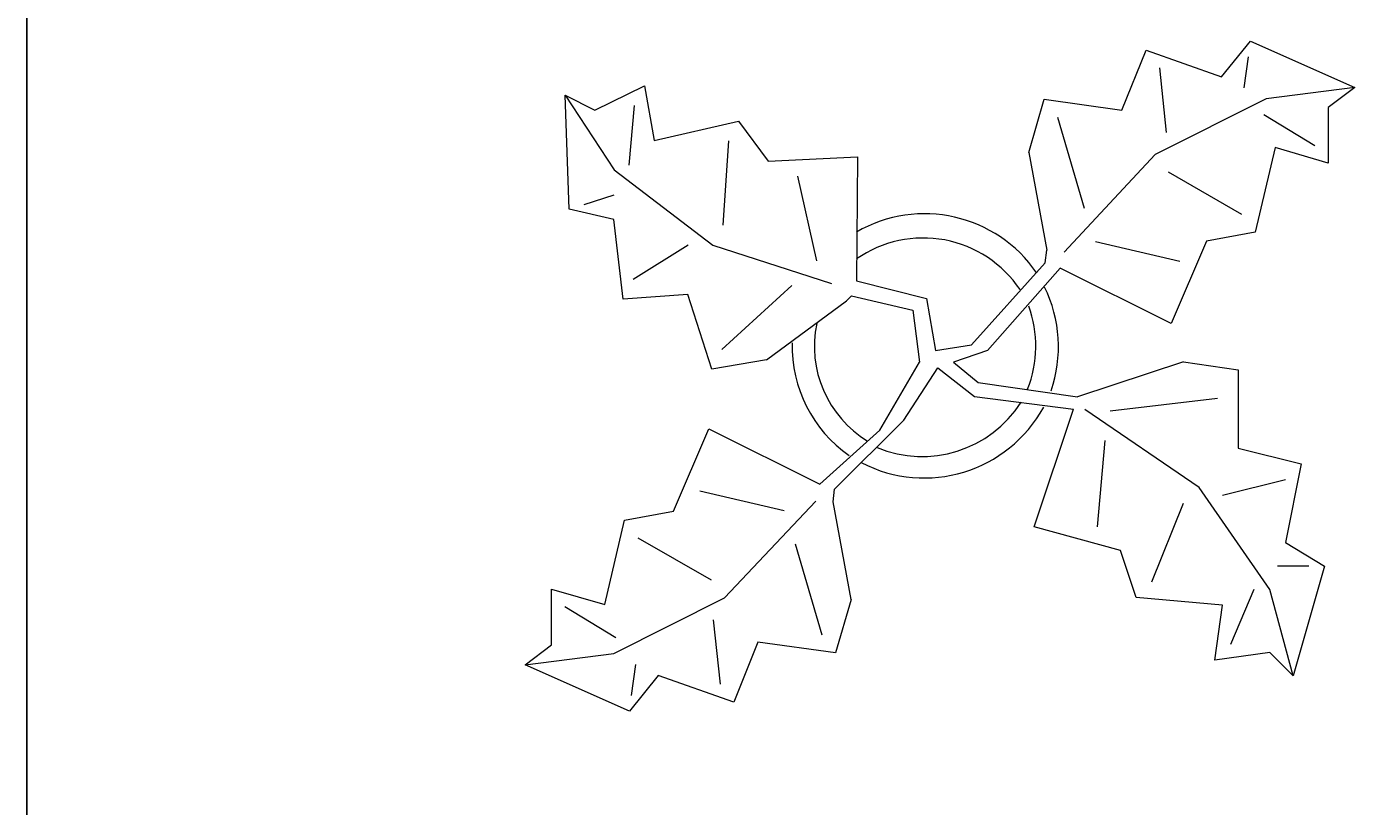
# Model space of a CAD drawing. Units: inches. Extents: x -301 to 715, y -607 to 364.
# Tile 54 of 141: x -205 to -164, y -260 to -237. Entities that reach past the tile are written whole.
import ezdxf

# ---------------------------------------------------------------- set-up
doc = ezdxf.new("R2010")
doc.units = ezdxf.units.IN
doc.header["$MEASUREMENT"] = 0
doc.layers.add('A-ANNO-DIMS', color=2, linetype='Continuous', lineweight=18)
doc.layers.add('L-PLNT', color=94, linetype='Continuous', lineweight=13)
doc.styles.get("Standard").update_dxf_attribs({"font": 'arial.ttf'})
doc.dimstyles.get("Standard").update_dxf_attribs({"dimtxt": 0.18, "dimasz": 0.18, "dimexe": 0.18, "dimexo": 0.0625, "dimgap": 0.09, "dimtad": 0, "dimtih": 1, "dimtoh": 1, "dimdec": 1, "dimzin": 0, "dimdsep": 46, "dimlunit": 4, "dimtxsty": 'Standard', "dimcen": 0.09, "dimclrd": 3, "dimclre": 4, "dimclrt": 6, "dimadec": 0, "dimazin": 0, "dimtfac": 1, "dimtdec": 1, "dimtofl": 0, "dimtmove": 0, "dimatfit": 3, "dimfxl": 1, "dimtfill": 2, "dimtfillclr": 51, "dimtolj": 1, "dimtzin": 0, "dimarcsym": 0})

# ---------------------------------------------------------------- blocks, each defined once
blk = doc.blocks.new('Plant - Rubber or Philodendron')
for p, q in [((8.8871, 10.7908), (9.9809, 13.4933)), ((9.9809, 13.4933), (13.3837, 12.301)), ((13.3837, 12.301), (14.68, 13.9039)), ((14.68, 13.9039), (19.3848, 11.8146)), ((14.5816, 13.2037), (14.3848, 11.8033)), ((10.5828, 12.6946), (10.8893, 9.7953)), ((-14.8639, 10.7964), (-12.6195, 11.8975)), ((-12.6195, 11.8975), (-12.1909, 9.4345)), ((19.3848, 11.8146), (15.3859, 11.3055)), ((19.3848, 11.8146), (18.1868, 10.9119)), ((-16.2005, 11.4774), (-13.9899, 8.1064)), ((-16.2005, 11.4774), (-14.8639, 10.7964)), ((-16.0159, 6.3329), (-16.2005, 11.4774)), ((-13.3174, 8.325), (-13.0735, 11.0065)), ((4.6914, 8.8812), (5.3859, 11.2828)), ((5.3859, 11.2828), (8.8871, 10.7908)), ((15.3859, 11.3055), (10.3916, 8.7942)), ((5.9878, 10.4842), (7.1971, 6.3869)), ((15.2875, 10.6053), (17.5907, 9.2105)), ((18.1868, 10.9119), (18.1925, 8.4119)), ((-12.1909, 9.4345), (-8.3829, 10.3)), ((-8.3829, 10.3), (-7.0549, 8.501)), ((-8.8369, 9.409), (-9.0894, 5.6095)), ((15.7909, 9.1065), (14.8995, 5.3044)), ((18.1925, 8.4119), (15.7909, 9.1065)), ((-7.0549, 8.501), (-3.0284, 8.6941)), ((-3.0284, 8.6941), (-3.0709, 3.1041)), ((4.6914, 8.8812), (5.5014, 4.4831)), ((10.3916, 8.7942), (6.2847, 4.4028)), ((-13.9899, 8.1064), (-9.5434, 4.7185)), ((14.2977, 6.1031), (10.9934, 7.9956)), ((-4.8529, 4.012), (-5.7184, 7.82)), ((-15.3434, 6.5514), (-13.9984, 6.9884)), ((-14.0069, 5.8704), (-16.0159, 6.3329)), ((-13.5868, 2.2894), (-14.0069, 5.8704)), ((7.7005, 4.8881), (11.5025, 3.9967)), ((12.7005, 4.8994), (11.1089, 1.1958)), ((14.8995, 5.3044), (12.7005, 4.8994)), ((-13.1329, 3.1804), (-10.6614, 4.727)), ((-9.5434, 4.7185), (-4.1917, 2.9888)), ((5.4346, 3.9146), (5.5014, 4.4831)), ((2.1141, 0.2298), (5.4346, 3.9146)), ((6.1032, 3.6844), (2.8262, -0.031)), ((11.1089, 1.1958), (6.1032, 3.6844)), ((-3.0709, 3.1041), (0.0797, 2.3163)), ((-10.6784, 2.491), (-13.5868, 2.2894)), ((-9.5858, -0.8715), (-10.6784, 2.491)), ((-9.1318, 0.0195), (-5.9793, 2.9025)), ((-3.5248, 2.2131), (-3.3011, 2.4355)), ((-3.3011, 2.4355), (-0.5306, 1.7947)), ((-7.1228, -0.443), (-3.5248, 2.2131)), ((0.0797, 2.3163), (0.4866, -0.031)), ((-0.5306, 1.7947), (-0.2255, -0.5527)), ((-0.5306, 1.7947), (-0.5306, 1.7947)), ((0.4866, -0.031), (2.1141, 0.2298)), ((-7.1228, -0.443), (-9.5858, -0.8715)), ((-2.019, -3.6148), (-0.2255, -0.5527)), ((2.8262, -0.031), (1.3003, -0.5527)), ((1.3003, -0.5527), (2.4193, -1.4655)), ((11.6605, -0.5413), (6.895, -2.1175)), ((11.6605, -0.5413), (14.1354, -0.8948)), ((-0.9375, -3.1608), (0.5883, -0.8135)), ((0.5883, -0.8135), (2.2447, -2.0916)), ((14.1354, -0.8948), (14.1354, -4.4304)), ((2.4193, -1.4655), (6.895, -2.1175)), ((2.2447, -2.0916), (6.7108, -2.6626)), ((8.3544, -2.7453), (13.1973, -2.1704)), ((4.943, -7.9659), (6.7108, -2.6626)), ((12.3677, -6.1981), (7.219, -2.6772)), ((-11.3237, -7.2629), (-9.7321, -3.5593)), ((-9.7321, -3.5593), (-4.7264, -6.0479)), ((-2.019, -3.6148), (-4.7264, -6.0479)), ((-4.0579, -6.2781), (-0.9375, -3.1608)), ((8.125, -4.0768), (7.7715, -7.9659)), ((14.1354, -4.4304), (16.9638, -5.1375)), ((16.9638, -5.1375), (16.2567, -8.673)), ((16.2567, -5.8446), (13.4283, -6.5517)), ((-6.3237, -7.2516), (-10.1257, -6.3602)), ((-4.1246, -6.8466), (-4.0579, -6.2781)), ((15.5496, -10.7943), (12.3677, -6.1981)), ((-13.5228, -7.6679), (-11.3237, -7.2629)), ((-9.0148, -11.1577), (-4.9047, -6.8122)), ((-3.3146, -11.2447), (-4.1246, -6.8466)), ((10.2463, -10.4408), (11.6605, -6.9053)), ((-14.4141, -11.4699), (-13.5228, -7.6679)), ((-12.921, -8.4665), (-9.6166, -10.359)), ((8.8321, -9.0266), (4.943, -7.9659)), ((-4.611, -12.8477), (-5.8203, -8.7504)), ((9.5392, -11.1479), (8.8321, -9.0266)), ((16.2567, -8.673), (18.0245, -9.7337)), ((17.3174, -9.7337), (15.9032, -9.7337)), ((18.0245, -9.7337), (16.6103, -14.6834)), ((-16.8157, -10.7754), (-14.4141, -11.4699)), ((-16.8101, -13.2754), (-16.8157, -10.7754)), ((14.8425, -10.7943), (13.7819, -13.2692)), ((16.6103, -14.6834), (15.5496, -10.7943)), ((-14.0091, -13.669), (-9.0148, -11.1577)), ((-3.3146, -11.2447), (-4.0092, -13.6463)), ((13.4283, -11.5015), (9.5392, -11.1479)), ((13.0748, -13.9763), (13.4283, -11.5015)), ((-13.9107, -12.9688), (-16.2139, -11.574)), ((-9.206, -15.0581), (-9.5126, -12.1588)), ((-18.008, -14.1781), (-16.8101, -13.2754)), ((-7.5103, -13.1543), (-8.6042, -15.8568)), ((-4.0092, -13.6463), (-7.5103, -13.1543)), ((-18.008, -14.1781), (-14.0091, -13.669)), ((15.5496, -13.6228), (13.0748, -13.9763)), ((16.6103, -14.6834), (15.5496, -13.6228)), ((-13.3032, -16.2674), (-18.008, -14.1781)), ((-13.2048, -15.5672), (-13.008, -14.1668)), ((-12.0069, -14.6645), (-13.3032, -16.2674)), ((-8.6042, -15.8568), (-12.0069, -14.6645))]:
    blk.add_line(p, q)
for centre, radius, start, end in [((0, 0), 6.1275, 34.37569, 120.1028), ((-0.0601, -0.2075), 5.2461, 33.82192, 124.9414), ((-0.098, 0.1364), 6.1288, 341.2017, 26.09184), ((-0.2664, 0.1682), 5.2775, 338.4094, 20.03007), ((0.0308, 0.1664), 5, 168.1647, 238.6725), ((0.0308, 0.1664), 6, 178.6147, 235.1169), ((-0.1102, 0.4886), 5.2883, 247.3711, 327.472), ((-0.0234, 0.3825), 6.1492, 242.5812, 331.2714)]:
    blk.add_arc(centre, radius, start, end)
blk = doc.blocks.new('*D146')
at = {"layer": 'A-ANNO-DIMS', "color": 4, "lineweight": -2, "transparency": 16777216}
for p, q in [((-204.603, -223.88), (-204.603, -296.865)), ((-143.603, -223.88), (-143.603, -296.865))]:
    blk.add_line(p, q, dxfattribs=at)
at = {"layer": 'A-ANNO-DIMS', "color": 3, "lineweight": -2, "transparency": 16777216}
for p, q in [((-204.423, -296.685), (-174.433, -296.685)), ((-143.783, -296.685), (-173.774, -296.685))]:
    blk.add_line(p, q, dxfattribs=at)
at = {"layer": 'A-ANNO-DIMS', "color": 3, "transparency": 16777216}
for points in [[(-204.423, -296.655), (-204.423, -296.715), (-204.603, -296.685)], [(-143.783, -296.655), (-143.783, -296.715), (-143.603, -296.685)]]:
    blk.add_solid(points, dxfattribs=at)
at = {"layer": 'Defpoints', "color": 0, "transparency": 16777216}
for p in [(-204.603, -223.818), (-143.603, -223.818), (-143.603, -296.685)]:
    blk.add_point(p, dxfattribs=at)
at = {"layer": 'A-ANNO-DIMS', "color": 6, "transparency": 16777216, "insert": (-174.103, -296.685), "char_height": 0.18, "attachment_point": 5, "bg_fill": 1, "box_fill_scale": 1.25, "bg_fill_color": 51, "bg_fill_transparency": 0}
blk.add_mtext('\\A1;5\'-1"', dxfattribs=at)

msp = doc.modelspace()

# ---------------------------------------------------------------- block references
at = {"layer": 'L-PLNT', "xscale": 0.6613521884636907, "yscale": 0.6613521884636907, "zscale": 0.6613521884636907}
msp.add_blockref('Plant - Rubber or Philodendron', (-177.848, -246.541), dxfattribs=at)

# ---------------------------------------------------------------- dimensions: what is measured, and where the dimension line sits
at = {"layer": 'A-ANNO-DIMS'}
dim = msp.add_linear_dim(base=(-143.603, -296.685), p1=(-204.603, -223.818), p2=(-143.603, -223.818), dimstyle='Standard', override={"dimdec": 1, "dimlfac": 1, "dimrnd": 0, "dimzin": 1, "dimdsep": 46, "dimlunit": 4, "dimfrac": 2}, dxfattribs=at)
dim.commit()
dim.dimension.update_dxf_attribs({"geometry": '*D146', "text_midpoint": (-174.103, -296.685)})

doc.saveas('drawing.dxf')
